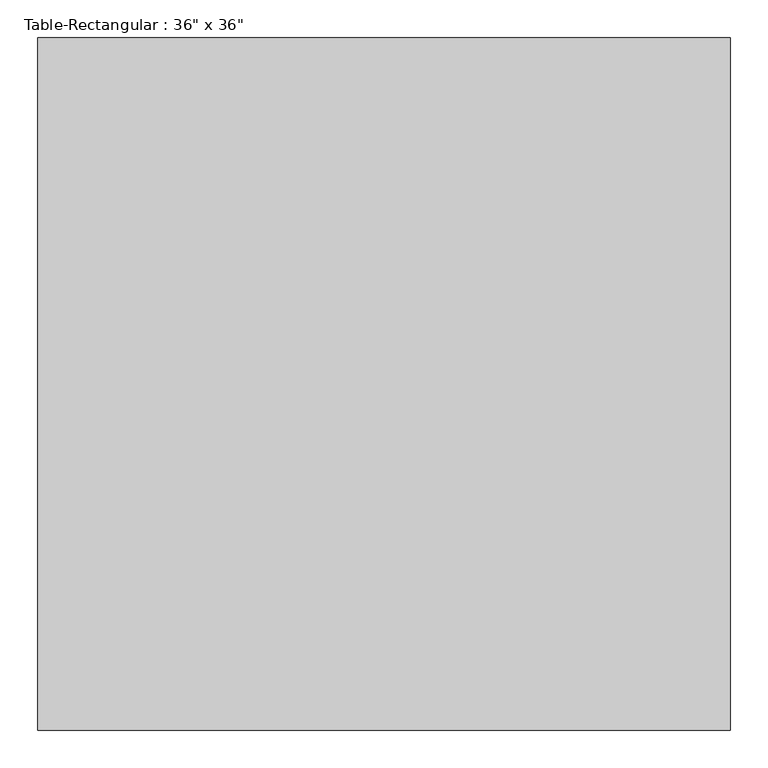
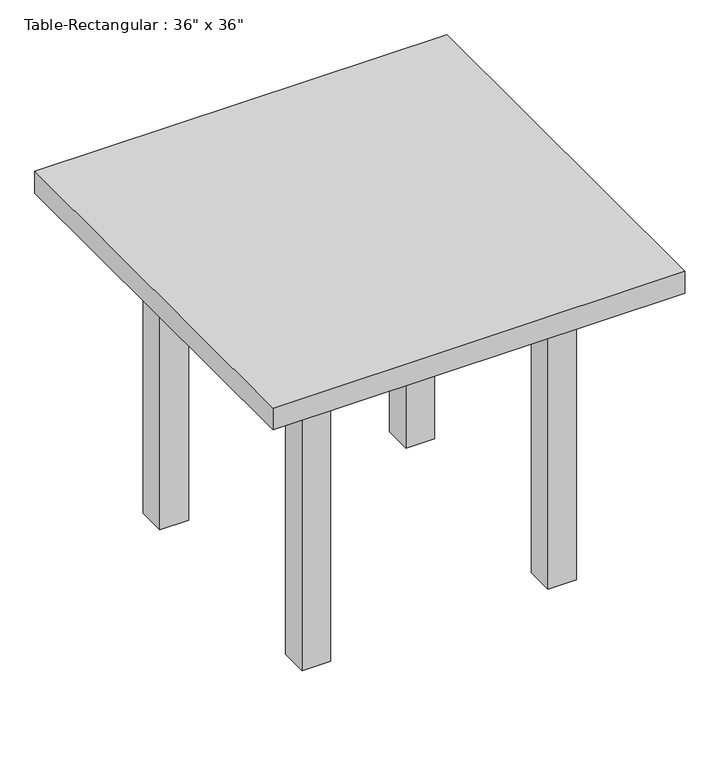
"""IFC4 building model written with IfcOpenShell, lengths in millimetres: furniture geometry."""

from ifc_helpers import new_model, si_unit, frame, origin, origin_with_axes, place, context, project, spatial, polyline, outline, extrude, source, transform, mapped, element, save


def furniture_4d44e21c(model_context):
    return source(origin(), model_context, "Body", "SweptSolid", [
        extrude(outline(polyline([(241.3, 266.7), (241.3, 241.3), (-241.3, 241.3), (-241.3, 266.7), (241.3, 266.7)])), frame((0.0, 0.0, 609.6), z_axis=(0.0, 0.0, 1.0), x_axis=(1.0, 0.0, 0.0)), (0.0, 0.0, 1.0), 101.6),
        extrude(outline(polyline([(241.3, -266.7), (-241.3, -266.7), (-241.3, -241.3), (241.3, -241.3), (241.3, -266.7)])), frame((0.0, 0.0, 609.6), z_axis=(0.0, 0.0, 1.0), x_axis=(1.0, 0.0, 0.0)), (0.0, 0.0, 1.0), 101.6),
        extrude(outline(polyline([(-254.0, -241.3), (-279.4, -241.3), (-279.4, 241.3), (-254.0, 241.3), (-254.0, -241.3)])), frame((0.0, 0.0, 609.6), z_axis=(0.0, 0.0, 1.0), x_axis=(1.0, 0.0, 0.0)), (0.0, 0.0, 1.0), 101.6),
        extrude(outline(polyline([(254.0, -241.3), (254.0, 241.3), (279.4, 241.3), (279.4, -241.3), (254.0, -241.3)])), frame((0.0, 0.0, 609.6), z_axis=(0.0, 0.0, 1.0), x_axis=(1.0, 0.0, 0.0)), (0.0, 0.0, 1.0), 101.6),
        extrude(outline(polyline([(457.2, 457.2), (457.2, -457.2), (-457.2, -457.2), (-457.2, 457.2), (457.2, 457.2)])), frame((0.0, 0.0, 711.2), z_axis=(0.0, 0.0, 1.0), x_axis=(1.0, 0.0, 0.0)), (0.0, 0.0, 1.0), 50.8),
        extrude(outline(polyline([(-241.3, 304.8), (-241.3, 241.3), (-304.8, 241.3), (-304.8, 304.8), (-241.3, 304.8)])), origin_with_axes(), (0.0, 0.0, 1.0), 711.2),
        extrude(outline(polyline([(241.3, 304.8), (304.8, 304.8), (304.8, 241.3), (241.3, 241.3), (241.3, 304.8)])), origin_with_axes(), (0.0, 0.0, 1.0), 711.2),
        extrude(outline(polyline([(-241.3, -304.8), (-304.8, -304.8), (-304.8, -241.3), (-241.3, -241.3), (-241.3, -304.8)])), origin_with_axes(), (0.0, 0.0, 1.0), 711.2),
        extrude(outline(polyline([(241.3, -304.8), (241.3, -241.3), (304.8, -241.3), (304.8, -304.8), (241.3, -304.8)])), origin_with_axes(), (0.0, 0.0, 1.0), 711.2),
    ])


if __name__ == "__main__":
    model = new_model("IFC4")
    model_context = context("Model", 3, world=origin())
    ifc_project = project(units=[si_unit("LENGTHUNIT", "METRE", prefix="MILLI")], contexts=[model_context])
    site = spatial("IfcSite", under=ifc_project)
    building = spatial("IfcBuilding", under=site)
    placement = place(None, origin())
    furniture_shape = furniture_4d44e21c(model_context)
    element("IfcFurniture", 1, ObjectType="Table-Rectangular : 36\" x 36\"", at=placement, inside=building, context=model_context, shape_type="MappedRepresentation", body=[
        mapped(furniture_shape, transform((0.0, 0.0, 0.0), x_axis=(1.0, 0.0, 0.0), y_axis=(0.0, 1.0, 0.0), z_axis=(0.0, 0.0, 1.0))),
    ])
    save(model, "model.ifc")

# Revit data of these elements
# Type "Table-Rectangular : 36\" x 36\""
#   Assembly Code = "E2020200"
#   Height = 2' - 6"
#   Length = 3' - 0"
#   Width = 3' - 0"
#   Base Material = Birch
#   Top Material = Copper
#   Default Elevation = 0
# Element 1 (IfcFurniture, "Table-Rectangular : 36\" x 36\"")
#   Materials on its faces: "Birch", "Copper"
# Materials
#   "Birch": class "Wood", colour RGB 224 178 126, transparency 0, Description = "Betula Alleghaniensis", Cost = 0
#   "Copper": class "Metal", colour RGB 0 0 0, transparency 0, Description = "Copper, matte finish", Cost = 0
